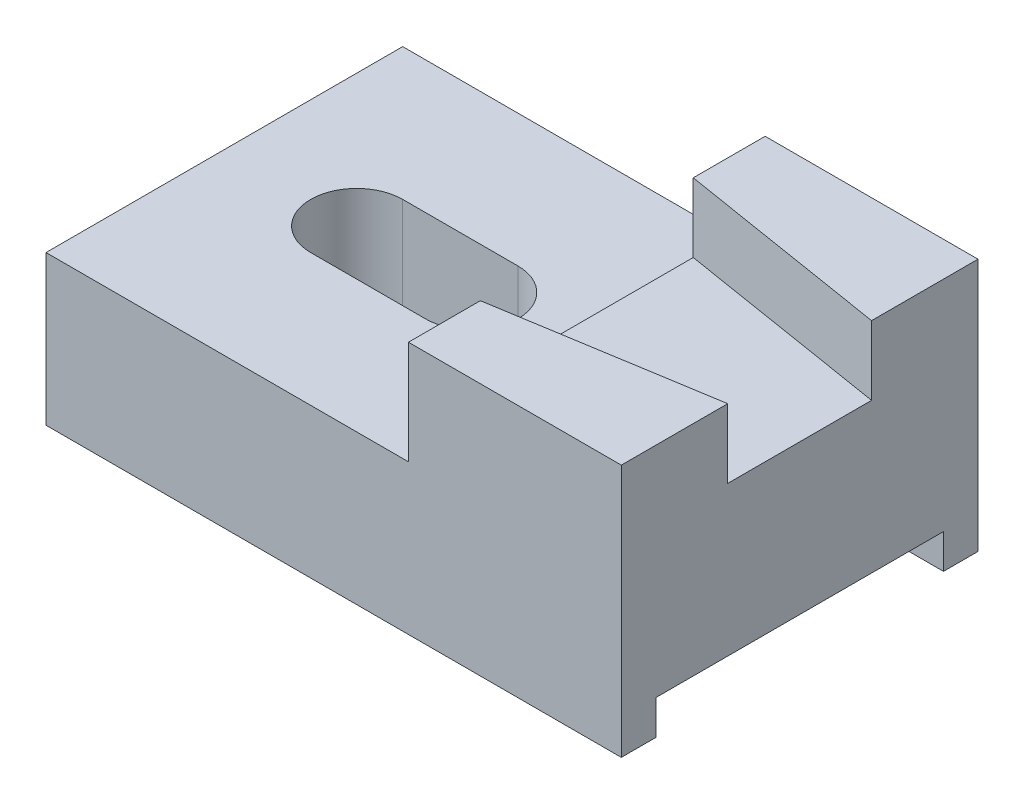
ISO-10303-21;
HEADER;
FILE_DESCRIPTION(('STEP AP214'),'2;1');
FILE_NAME('part.step','',(''),(''),'','','');
FILE_SCHEMA(('AUTOMOTIVE_DESIGN { 1 0 10303 214 1 1 1 1 }'));
ENDSEC;
DATA;
#1=APPLICATION_CONTEXT('core data for automotive mechanical design processes');
#2=APPLICATION_PROTOCOL_DEFINITION('international standard','automotive_design',2000,#1);
#3=PRODUCT_CONTEXT('',#1,'mechanical');
#4=PRODUCT('Part','Part','',(#3));
#5=PRODUCT_RELATED_PRODUCT_CATEGORY('part','',(#4));
#6=PRODUCT_DEFINITION_FORMATION('','',#4);
#7=PRODUCT_DEFINITION_CONTEXT('part definition',#1,'design');
#8=PRODUCT_DEFINITION('design','',#6,#7);
#9=PRODUCT_DEFINITION_SHAPE('','',#8);
#10=(LENGTH_UNIT() NAMED_UNIT(*) SI_UNIT(.MILLI.,.METRE.));
#11=(NAMED_UNIT(*) PLANE_ANGLE_UNIT() SI_UNIT($,.RADIAN.));
#12=(NAMED_UNIT(*) SI_UNIT($,.STERADIAN.) SOLID_ANGLE_UNIT());
#13=UNCERTAINTY_MEASURE_WITH_UNIT(LENGTH_MEASURE(1.E-05),#10,'distance_accuracy_value','');
#14=(GEOMETRIC_REPRESENTATION_CONTEXT(3) GLOBAL_UNCERTAINTY_ASSIGNED_CONTEXT((#13)) GLOBAL_UNIT_ASSIGNED_CONTEXT((#10,
#11,#12)) REPRESENTATION_CONTEXT('',''));
#15=CARTESIAN_POINT('',(0.,0.,0.));
#16=DIRECTION('',(0.,0.,1.));
#17=DIRECTION('',(1.,0.,0.));
#18=AXIS2_PLACEMENT_3D('',#15,#16,#17);
#19=CARTESIAN_POINT('',(100.,0.,31.));
#20=DIRECTION('',(0.,1.,0.));
#21=DIRECTION('',(0.,0.,1.));
#22=AXIS2_PLACEMENT_3D('',#19,#20,#21);
#23=PLANE('',#22);
#24=DIRECTION('',(-1.,0.,0.));
#25=VECTOR('',#24,1.);
#26=CARTESIAN_POINT('',(100.,0.,-25.));
#27=LINE('',#26,#25);
#28=CARTESIAN_POINT('',(100.,0.,-25.));
#29=VERTEX_POINT('',#28);
#30=CARTESIAN_POINT('',(0.,0.,-25.));
#31=VERTEX_POINT('',#30);
#32=EDGE_CURVE('E166',#29,#31,#27,.T.);
#33=ORIENTED_EDGE('',*,*,#32,.T.);
#34=DIRECTION('',(0.,0.,-1.));
#35=VECTOR('',#34,1.);
#36=CARTESIAN_POINT('',(0.,0.,31.));
#37=LINE('',#36,#35);
#38=CARTESIAN_POINT('',(0.,0.,-31.));
#39=VERTEX_POINT('',#38);
#40=EDGE_CURVE('E265',#31,#39,#37,.T.);
#41=ORIENTED_EDGE('',*,*,#40,.T.);
#42=DIRECTION('',(1.,0.,0.));
#43=VECTOR('',#42,1.);
#44=CARTESIAN_POINT('',(100.,0.,-31.));
#45=LINE('',#44,#43);
#46=CARTESIAN_POINT('',(100.,0.,-31.));
#47=VERTEX_POINT('',#46);
#48=EDGE_CURVE('E241',#39,#47,#45,.T.);
#49=ORIENTED_EDGE('',*,*,#48,.T.);
#50=DIRECTION('',(0.,0.,-1.));
#51=VECTOR('',#50,1.);
#52=CARTESIAN_POINT('',(100.,0.,31.));
#53=LINE('',#52,#51);
#54=EDGE_CURVE('E291',#29,#47,#53,.T.);
#55=ORIENTED_EDGE('',*,*,#54,.F.);
#56=EDGE_LOOP('',(#33,#41,#49,#55));
#57=FACE_BOUND('',#56,.T.);
#58=ADVANCED_FACE('F39',(#57),#23,.F.);
#59=DIRECTION('',(-1.,0.,0.));
#60=VECTOR('',#59,1.);
#61=CARTESIAN_POINT('',(100.,0.,25.));
#62=LINE('',#61,#60);
#63=CARTESIAN_POINT('',(100.,0.,25.));
#64=VERTEX_POINT('',#63);
#65=CARTESIAN_POINT('',(0.,0.,25.));
#66=VERTEX_POINT('',#65);
#67=EDGE_CURVE('E52',#64,#66,#62,.T.);
#68=ORIENTED_EDGE('',*,*,#67,.F.);
#69=CARTESIAN_POINT('',(100.,0.,31.));
#70=VERTEX_POINT('',#69);
#71=EDGE_CURVE('E46',#70,#64,#53,.T.);
#72=ORIENTED_EDGE('',*,*,#71,.F.);
#73=DIRECTION('',(1.,0.,0.));
#74=VECTOR('',#73,1.);
#75=CARTESIAN_POINT('',(100.,0.,31.));
#76=LINE('',#75,#74);
#77=CARTESIAN_POINT('',(0.,0.,31.));
#78=VERTEX_POINT('',#77);
#79=EDGE_CURVE('E246',#78,#70,#76,.T.);
#80=ORIENTED_EDGE('',*,*,#79,.F.);
#81=EDGE_CURVE('E280',#78,#66,#37,.T.);
#82=ORIENTED_EDGE('',*,*,#81,.T.);
#83=EDGE_LOOP('',(#68,#72,#80,#82));
#84=FACE_BOUND('',#83,.T.);
#85=ADVANCED_FACE('F341',(#84),#23,.F.);
#86=CARTESIAN_POINT('',(100.,44.,31.));
#87=DIRECTION('',(-1.,0.,0.));
#88=DIRECTION('',(0.,0.,1.));
#89=AXIS2_PLACEMENT_3D('',#86,#87,#88);
#90=PLANE('',#89);
#91=DIRECTION('',(0.,1.,0.));
#92=VECTOR('',#91,1.);
#93=CARTESIAN_POINT('',(100.,0.,-25.));
#94=LINE('',#93,#92);
#95=CARTESIAN_POINT('',(100.,5.99999999999997,-25.));
#96=VERTEX_POINT('',#95);
#97=EDGE_CURVE('E162',#29,#96,#94,.T.);
#98=ORIENTED_EDGE('',*,*,#97,.F.);
#99=ORIENTED_EDGE('',*,*,#54,.T.);
#100=DIRECTION('',(0.,1.,0.));
#101=VECTOR('',#100,1.);
#102=CARTESIAN_POINT('',(100.,44.,-31.));
#103=LINE('',#102,#101);
#104=CARTESIAN_POINT('',(100.,44.,-31.));
#105=VERTEX_POINT('',#104);
#106=EDGE_CURVE('E264',#47,#105,#103,.T.);
#107=ORIENTED_EDGE('',*,*,#106,.T.);
#108=DIRECTION('',(0.,0.,-1.));
#109=VECTOR('',#108,1.);
#110=CARTESIAN_POINT('',(100.,44.,31.));
#111=LINE('',#110,#109);
#112=CARTESIAN_POINT('',(100.,44.,-12.5));
#113=VERTEX_POINT('',#112);
#114=EDGE_CURVE('E287',#113,#105,#111,.T.);
#115=ORIENTED_EDGE('',*,*,#114,.F.);
#116=DIRECTION('',(0.,1.,0.));
#117=VECTOR('',#116,1.);
#118=CARTESIAN_POINT('',(100.,32.,-12.5));
#119=LINE('',#118,#117);
#120=CARTESIAN_POINT('',(100.,32.,-12.5));
#121=VERTEX_POINT('',#120);
#122=EDGE_CURVE('E217',#121,#113,#119,.T.);
#123=ORIENTED_EDGE('',*,*,#122,.F.);
#124=DIRECTION('',(0.,0.,-1.));
#125=VECTOR('',#124,1.);
#126=CARTESIAN_POINT('',(100.,32.,-12.5));
#127=LINE('',#126,#125);
#128=CARTESIAN_POINT('',(100.,32.,12.5));
#129=VERTEX_POINT('',#128);
#130=EDGE_CURVE('E215',#129,#121,#127,.T.);
#131=ORIENTED_EDGE('',*,*,#130,.F.);
#132=DIRECTION('',(0.,1.,0.));
#133=VECTOR('',#132,1.);
#134=CARTESIAN_POINT('',(100.,32.,12.5));
#135=LINE('',#134,#133);
#136=CARTESIAN_POINT('',(100.,44.,12.5));
#137=VERTEX_POINT('',#136);
#138=EDGE_CURVE('E222',#129,#137,#135,.T.);
#139=ORIENTED_EDGE('',*,*,#138,.T.);
#140=CARTESIAN_POINT('',(100.,44.,31.));
#141=VERTEX_POINT('',#140);
#142=EDGE_CURVE('E292',#141,#137,#111,.T.);
#143=ORIENTED_EDGE('',*,*,#142,.F.);
#144=DIRECTION('',(0.,1.,0.));
#145=VECTOR('',#144,1.);
#146=CARTESIAN_POINT('',(100.,44.,31.));
#147=LINE('',#146,#145);
#148=EDGE_CURVE('E253',#70,#141,#147,.T.);
#149=ORIENTED_EDGE('',*,*,#148,.F.);
#150=ORIENTED_EDGE('',*,*,#71,.T.);
#151=DIRECTION('',(0.,-1.,0.));
#152=VECTOR('',#151,1.);
#153=CARTESIAN_POINT('',(100.,5.99999999999997,25.));
#154=LINE('',#153,#152);
#155=CARTESIAN_POINT('',(100.,5.99999999999997,25.));
#156=VERTEX_POINT('',#155);
#157=EDGE_CURVE('E186',#156,#64,#154,.T.);
#158=ORIENTED_EDGE('',*,*,#157,.F.);
#159=DIRECTION('',(0.,0.,1.));
#160=VECTOR('',#159,1.);
#161=CARTESIAN_POINT('',(100.,5.99999999999997,-25.));
#162=LINE('',#161,#160);
#163=EDGE_CURVE('E175',#96,#156,#162,.T.);
#164=ORIENTED_EDGE('',*,*,#163,.F.);
#165=EDGE_LOOP('',(#98,#99,#107,#115,#123,#131,#139,#143,#149,#150,#158,#164));
#166=FACE_BOUND('',#165,.T.);
#167=ADVANCED_FACE('F183',(#166),#90,.F.);
#168=CARTESIAN_POINT('',(0.,0.,31.));
#169=DIRECTION('',(1.,0.,0.));
#170=DIRECTION('',(0.,1.,0.));
#171=AXIS2_PLACEMENT_3D('',#168,#169,#170);
#172=PLANE('',#171);
#173=DIRECTION('',(0.,1.,0.));
#174=VECTOR('',#173,1.);
#175=CARTESIAN_POINT('',(0.,0.,-25.));
#176=LINE('',#175,#174);
#177=CARTESIAN_POINT('',(0.,5.99999999999999,-25.));
#178=VERTEX_POINT('',#177);
#179=EDGE_CURVE('E193',#31,#178,#176,.T.);
#180=ORIENTED_EDGE('',*,*,#179,.T.);
#181=DIRECTION('',(0.,0.,1.));
#182=VECTOR('',#181,1.);
#183=CARTESIAN_POINT('',(0.,5.99999999999999,-25.));
#184=LINE('',#183,#182);
#185=CARTESIAN_POINT('',(0.,5.99999999999999,25.));
#186=VERTEX_POINT('',#185);
#187=EDGE_CURVE('E177',#178,#186,#184,.T.);
#188=ORIENTED_EDGE('',*,*,#187,.T.);
#189=DIRECTION('',(0.,-1.,0.));
#190=VECTOR('',#189,1.);
#191=CARTESIAN_POINT('',(0.,5.99999999999999,25.));
#192=LINE('',#191,#190);
#193=EDGE_CURVE('E173',#186,#66,#192,.T.);
#194=ORIENTED_EDGE('',*,*,#193,.T.);
#195=ORIENTED_EDGE('',*,*,#81,.F.);
#196=DIRECTION('',(0.,-1.,0.));
#197=VECTOR('',#196,1.);
#198=CARTESIAN_POINT('',(0.,0.,31.));
#199=LINE('',#198,#197);
#200=CARTESIAN_POINT('',(0.,26.,31.));
#201=VERTEX_POINT('',#200);
#202=EDGE_CURVE('E257',#201,#78,#199,.T.);
#203=ORIENTED_EDGE('',*,*,#202,.F.);
#204=DIRECTION('',(0.,0.,-1.));
#205=VECTOR('',#204,1.);
#206=CARTESIAN_POINT('',(0.,26.,31.));
#207=LINE('',#206,#205);
#208=CARTESIAN_POINT('',(0.,26.,-31.));
#209=VERTEX_POINT('',#208);
#210=EDGE_CURVE('E278',#201,#209,#207,.T.);
#211=ORIENTED_EDGE('',*,*,#210,.T.);
#212=DIRECTION('',(0.,-1.,0.));
#213=VECTOR('',#212,1.);
#214=CARTESIAN_POINT('',(0.,0.,-31.));
#215=LINE('',#214,#213);
#216=EDGE_CURVE('E252',#209,#39,#215,.T.);
#217=ORIENTED_EDGE('',*,*,#216,.T.);
#218=ORIENTED_EDGE('',*,*,#40,.F.);
#219=EDGE_LOOP('',(#180,#188,#194,#195,#203,#211,#217,#218));
#220=FACE_BOUND('',#219,.T.);
#221=ADVANCED_FACE('F308',(#220),#172,.F.);
#222=CARTESIAN_POINT('',(23.,-36.,0.));
#223=DIRECTION('',(0.,1.,0.));
#224=DIRECTION('',(0.,0.,1.));
#225=AXIS2_PLACEMENT_3D('',#222,#223,#224);
#226=CYLINDRICAL_SURFACE('',#225,8.);
#227=CARTESIAN_POINT('',(23.,5.99999999999998,0.));
#228=DIRECTION('',(0.,-1.,0.));
#229=DIRECTION('',(1.,0.,0.));
#230=AXIS2_PLACEMENT_3D('',#227,#228,#229);
#231=CIRCLE('',#230,8.);
#232=CARTESIAN_POINT('',(23.,5.99999999999998,-8.));
#233=VERTEX_POINT('',#232);
#234=CARTESIAN_POINT('',(23.,5.99999999999998,8.));
#235=VERTEX_POINT('',#234);
#236=EDGE_CURVE('E58',#233,#235,#231,.F.);
#237=ORIENTED_EDGE('',*,*,#236,.F.);
#238=DIRECTION('',(0.,1.,0.));
#239=VECTOR('',#238,1.);
#240=CARTESIAN_POINT('',(23.,-36.,-8.));
#241=LINE('',#240,#239);
#242=CARTESIAN_POINT('',(23.,26.,-8.));
#243=VERTEX_POINT('',#242);
#244=EDGE_CURVE('E238',#233,#243,#241,.T.);
#245=ORIENTED_EDGE('',*,*,#244,.T.);
#246=CARTESIAN_POINT('',(23.,26.,0.));
#247=DIRECTION('',(0.,1.,0.));
#248=DIRECTION('',(0.,0.,1.));
#249=AXIS2_PLACEMENT_3D('',#246,#247,#248);
#250=CIRCLE('',#249,8.);
#251=CARTESIAN_POINT('',(23.,26.,8.));
#252=VERTEX_POINT('',#251);
#253=EDGE_CURVE('E219',#243,#252,#250,.T.);
#254=ORIENTED_EDGE('',*,*,#253,.T.);
#255=DIRECTION('',(0.,1.,0.));
#256=VECTOR('',#255,1.);
#257=CARTESIAN_POINT('',(23.,-36.,8.));
#258=LINE('',#257,#256);
#259=EDGE_CURVE('E239',#235,#252,#258,.T.);
#260=ORIENTED_EDGE('',*,*,#259,.F.);
#261=EDGE_LOOP('',(#237,#245,#254,#260));
#262=FACE_BOUND('',#261,.T.);
#263=ADVANCED_FACE('F361',(#262),#226,.F.);
#264=CARTESIAN_POINT('',(23.,-36.,-8.));
#265=DIRECTION('',(0.,0.,-1.));
#266=DIRECTION('',(-1.,0.,0.));
#267=AXIS2_PLACEMENT_3D('',#264,#265,#266);
#268=PLANE('',#267);
#269=DIRECTION('',(-1.,0.,0.));
#270=VECTOR('',#269,1.);
#271=CARTESIAN_POINT('',(23.,5.99999999999998,-8.));
#272=LINE('',#271,#270);
#273=CARTESIAN_POINT('',(43.,5.99999999999998,-8.));
#274=VERTEX_POINT('',#273);
#275=EDGE_CURVE('E200',#274,#233,#272,.T.);
#276=ORIENTED_EDGE('',*,*,#275,.F.);
#277=DIRECTION('',(0.,1.,0.));
#278=VECTOR('',#277,1.);
#279=CARTESIAN_POINT('',(43.,-36.,-8.));
#280=LINE('',#279,#278);
#281=CARTESIAN_POINT('',(43.,26.,-8.));
#282=VERTEX_POINT('',#281);
#283=EDGE_CURVE('E245',#274,#282,#280,.T.);
#284=ORIENTED_EDGE('',*,*,#283,.T.);
#285=DIRECTION('',(-1.,0.,0.));
#286=VECTOR('',#285,1.);
#287=CARTESIAN_POINT('',(23.,26.,-8.));
#288=LINE('',#287,#286);
#289=EDGE_CURVE('E237',#282,#243,#288,.T.);
#290=ORIENTED_EDGE('',*,*,#289,.T.);
#291=ORIENTED_EDGE('',*,*,#244,.F.);
#292=EDGE_LOOP('',(#276,#284,#290,#291));
#293=FACE_BOUND('',#292,.T.);
#294=ADVANCED_FACE('F377',(#293),#268,.F.);
#295=CARTESIAN_POINT('',(43.,-36.,0.));
#296=DIRECTION('',(0.,1.,0.));
#297=DIRECTION('',(0.,0.,1.));
#298=AXIS2_PLACEMENT_3D('',#295,#296,#297);
#299=CYLINDRICAL_SURFACE('',#298,8.);
#300=CARTESIAN_POINT('',(43.,5.99999999999998,0.));
#301=DIRECTION('',(0.,-1.,0.));
#302=DIRECTION('',(1.,0.,0.));
#303=AXIS2_PLACEMENT_3D('',#300,#301,#302);
#304=CIRCLE('',#303,8.);
#305=CARTESIAN_POINT('',(43.,5.99999999999998,8.));
#306=VERTEX_POINT('',#305);
#307=EDGE_CURVE('E182',#306,#274,#304,.F.);
#308=ORIENTED_EDGE('',*,*,#307,.F.);
#309=DIRECTION('',(0.,1.,0.));
#310=VECTOR('',#309,1.);
#311=CARTESIAN_POINT('',(43.,-36.,8.));
#312=LINE('',#311,#310);
#313=CARTESIAN_POINT('',(43.,26.,8.));
#314=VERTEX_POINT('',#313);
#315=EDGE_CURVE('E242',#306,#314,#312,.T.);
#316=ORIENTED_EDGE('',*,*,#315,.T.);
#317=CARTESIAN_POINT('',(43.,26.,0.));
#318=DIRECTION('',(0.,1.,0.));
#319=DIRECTION('',(0.,0.,1.));
#320=AXIS2_PLACEMENT_3D('',#317,#318,#319);
#321=CIRCLE('',#320,8.);
#322=EDGE_CURVE('E231',#314,#282,#321,.T.);
#323=ORIENTED_EDGE('',*,*,#322,.T.);
#324=ORIENTED_EDGE('',*,*,#283,.F.);
#325=EDGE_LOOP('',(#308,#316,#323,#324));
#326=FACE_BOUND('',#325,.T.);
#327=ADVANCED_FACE('F383',(#326),#299,.F.);
#328=CARTESIAN_POINT('',(23.,-36.,8.));
#329=DIRECTION('',(0.,0.,1.));
#330=DIRECTION('',(1.,0.,0.));
#331=AXIS2_PLACEMENT_3D('',#328,#329,#330);
#332=PLANE('',#331);
#333=DIRECTION('',(1.,0.,0.));
#334=VECTOR('',#333,1.);
#335=CARTESIAN_POINT('',(23.,5.99999999999998,8.));
#336=LINE('',#335,#334);
#337=EDGE_CURVE('E11',#235,#306,#336,.T.);
#338=ORIENTED_EDGE('',*,*,#337,.F.);
#339=ORIENTED_EDGE('',*,*,#259,.T.);
#340=DIRECTION('',(1.,0.,0.));
#341=VECTOR('',#340,1.);
#342=CARTESIAN_POINT('',(23.,26.,8.));
#343=LINE('',#342,#341);
#344=EDGE_CURVE('E227',#252,#314,#343,.T.);
#345=ORIENTED_EDGE('',*,*,#344,.T.);
#346=ORIENTED_EDGE('',*,*,#315,.F.);
#347=EDGE_LOOP('',(#338,#339,#345,#346));
#348=FACE_BOUND('',#347,.T.);
#349=ADVANCED_FACE('F381',(#348),#332,.F.);
#350=CARTESIAN_POINT('',(63.,44.,31.));
#351=DIRECTION('',(0.,-1.,0.));
#352=DIRECTION('',(1.,0.,0.));
#353=AXIS2_PLACEMENT_3D('',#350,#351,#352);
#354=PLANE('',#353);
#355=DIRECTION('',(0.,0.,-1.));
#356=VECTOR('',#355,1.);
#357=CARTESIAN_POINT('',(63.,44.,31.));
#358=LINE('',#357,#356);
#359=CARTESIAN_POINT('',(63.,44.,-18.5));
#360=VERTEX_POINT('',#359);
#361=CARTESIAN_POINT('',(63.,44.,-31.));
#362=VERTEX_POINT('',#361);
#363=EDGE_CURVE('E288',#360,#362,#358,.T.);
#364=ORIENTED_EDGE('',*,*,#363,.F.);
#365=DIRECTION('',(-0.987105477747585,0.,-0.160071158553662));
#366=VECTOR('',#365,1.);
#367=CARTESIAN_POINT('',(63.,44.,-18.5));
#368=LINE('',#367,#366);
#369=EDGE_CURVE('E205',#113,#360,#368,.T.);
#370=ORIENTED_EDGE('',*,*,#369,.F.);
#371=ORIENTED_EDGE('',*,*,#114,.T.);
#372=DIRECTION('',(-1.,0.,0.));
#373=VECTOR('',#372,1.);
#374=CARTESIAN_POINT('',(63.,44.,-31.));
#375=LINE('',#374,#373);
#376=EDGE_CURVE('E268',#105,#362,#375,.T.);
#377=ORIENTED_EDGE('',*,*,#376,.T.);
#378=EDGE_LOOP('',(#364,#370,#371,#377));
#379=FACE_BOUND('',#378,.T.);
#380=ADVANCED_FACE('F325',(#379),#354,.F.);
#381=ORIENTED_EDGE('',*,*,#142,.T.);
#382=DIRECTION('',(0.987105477747585,0.,-0.160071158553662));
#383=VECTOR('',#382,1.);
#384=CARTESIAN_POINT('',(63.,44.,18.5));
#385=LINE('',#384,#383);
#386=CARTESIAN_POINT('',(63.,44.,18.5));
#387=VERTEX_POINT('',#386);
#388=EDGE_CURVE('E206',#387,#137,#385,.T.);
#389=ORIENTED_EDGE('',*,*,#388,.F.);
#390=CARTESIAN_POINT('',(63.,44.,31.));
#391=VERTEX_POINT('',#390);
#392=EDGE_CURVE('E290',#391,#387,#358,.T.);
#393=ORIENTED_EDGE('',*,*,#392,.F.);
#394=DIRECTION('',(-1.,0.,0.));
#395=VECTOR('',#394,1.);
#396=CARTESIAN_POINT('',(63.,44.,31.));
#397=LINE('',#396,#395);
#398=EDGE_CURVE('E255',#141,#391,#397,.T.);
#399=ORIENTED_EDGE('',*,*,#398,.F.);
#400=EDGE_LOOP('',(#381,#389,#393,#399));
#401=FACE_BOUND('',#400,.T.);
#402=ADVANCED_FACE('F339',(#401),#354,.F.);
#403=CARTESIAN_POINT('',(63.,26.,31.));
#404=DIRECTION('',(1.,0.,0.));
#405=DIRECTION('',(0.,1.,0.));
#406=AXIS2_PLACEMENT_3D('',#403,#404,#405);
#407=PLANE('',#406);
#408=DIRECTION('',(0.,0.,1.));
#409=VECTOR('',#408,1.);
#410=CARTESIAN_POINT('',(63.,32.,-18.5));
#411=LINE('',#410,#409);
#412=CARTESIAN_POINT('',(63.,32.,-18.5));
#413=VERTEX_POINT('',#412);
#414=CARTESIAN_POINT('',(63.,32.,18.5));
#415=VERTEX_POINT('',#414);
#416=EDGE_CURVE('E202',#413,#415,#411,.T.);
#417=ORIENTED_EDGE('',*,*,#416,.F.);
#418=DIRECTION('',(0.,1.,0.));
#419=VECTOR('',#418,1.);
#420=CARTESIAN_POINT('',(63.,32.,-18.5));
#421=LINE('',#420,#419);
#422=EDGE_CURVE('E214',#413,#360,#421,.T.);
#423=ORIENTED_EDGE('',*,*,#422,.T.);
#424=ORIENTED_EDGE('',*,*,#363,.T.);
#425=DIRECTION('',(0.,-1.,0.));
#426=VECTOR('',#425,1.);
#427=CARTESIAN_POINT('',(63.,26.,-31.));
#428=LINE('',#427,#426);
#429=CARTESIAN_POINT('',(63.,26.,-31.));
#430=VERTEX_POINT('',#429);
#431=EDGE_CURVE('E271',#362,#430,#428,.T.);
#432=ORIENTED_EDGE('',*,*,#431,.T.);
#433=DIRECTION('',(0.,0.,-1.));
#434=VECTOR('',#433,1.);
#435=CARTESIAN_POINT('',(63.,26.,31.));
#436=LINE('',#435,#434);
#437=CARTESIAN_POINT('',(63.,26.,31.));
#438=VERTEX_POINT('',#437);
#439=EDGE_CURVE('E285',#438,#430,#436,.T.);
#440=ORIENTED_EDGE('',*,*,#439,.F.);
#441=DIRECTION('',(0.,-1.,0.));
#442=VECTOR('',#441,1.);
#443=CARTESIAN_POINT('',(63.,26.,31.));
#444=LINE('',#443,#442);
#445=EDGE_CURVE('E258',#391,#438,#444,.T.);
#446=ORIENTED_EDGE('',*,*,#445,.F.);
#447=ORIENTED_EDGE('',*,*,#392,.T.);
#448=DIRECTION('',(0.,1.,0.));
#449=VECTOR('',#448,1.);
#450=CARTESIAN_POINT('',(63.,32.,18.5));
#451=LINE('',#450,#449);
#452=EDGE_CURVE('E221',#415,#387,#451,.T.);
#453=ORIENTED_EDGE('',*,*,#452,.F.);
#454=EDGE_LOOP('',(#417,#423,#424,#432,#440,#446,#447,#453));
#455=FACE_BOUND('',#454,.T.);
#456=ADVANCED_FACE('F320',(#455),#407,.F.);
#457=CARTESIAN_POINT('',(0.,26.,31.));
#458=DIRECTION('',(0.,-1.,0.));
#459=DIRECTION('',(0.,0.,-1.));
#460=AXIS2_PLACEMENT_3D('',#457,#458,#459);
#461=PLANE('',#460);
#462=ORIENTED_EDGE('',*,*,#344,.F.);
#463=ORIENTED_EDGE('',*,*,#253,.F.);
#464=ORIENTED_EDGE('',*,*,#289,.F.);
#465=ORIENTED_EDGE('',*,*,#322,.F.);
#466=EDGE_LOOP('',(#462,#463,#464,#465));
#467=FACE_BOUND('',#466,.T.);
#468=DIRECTION('',(-1.,0.,0.));
#469=VECTOR('',#468,1.);
#470=CARTESIAN_POINT('',(0.,26.,-31.));
#471=LINE('',#470,#469);
#472=EDGE_CURVE('E272',#430,#209,#471,.T.);
#473=ORIENTED_EDGE('',*,*,#472,.T.);
#474=ORIENTED_EDGE('',*,*,#210,.F.);
#475=DIRECTION('',(-1.,0.,0.));
#476=VECTOR('',#475,1.);
#477=CARTESIAN_POINT('',(0.,26.,31.));
#478=LINE('',#477,#476);
#479=EDGE_CURVE('E256',#438,#201,#478,.T.);
#480=ORIENTED_EDGE('',*,*,#479,.F.);
#481=ORIENTED_EDGE('',*,*,#439,.T.);
#482=EDGE_LOOP('',(#473,#474,#480,#481));
#483=FACE_BOUND('',#482,.T.);
#484=ADVANCED_FACE('F313',(#467,#483),#461,.F.);
#485=CARTESIAN_POINT('',(0.,0.,31.));
#486=DIRECTION('',(0.,0.,-1.));
#487=DIRECTION('',(-1.,0.,0.));
#488=AXIS2_PLACEMENT_3D('',#485,#486,#487);
#489=PLANE('',#488);
#490=ORIENTED_EDGE('',*,*,#79,.T.);
#491=ORIENTED_EDGE('',*,*,#148,.T.);
#492=ORIENTED_EDGE('',*,*,#398,.T.);
#493=ORIENTED_EDGE('',*,*,#445,.T.);
#494=ORIENTED_EDGE('',*,*,#479,.T.);
#495=ORIENTED_EDGE('',*,*,#202,.T.);
#496=EDGE_LOOP('',(#490,#491,#492,#493,#494,#495));
#497=FACE_BOUND('',#496,.T.);
#498=ADVANCED_FACE('F338',(#497),#489,.F.);
#499=CARTESIAN_POINT('',(0.,0.,-31.));
#500=DIRECTION('',(0.,0.,-1.));
#501=DIRECTION('',(-1.,0.,0.));
#502=AXIS2_PLACEMENT_3D('',#499,#500,#501);
#503=PLANE('',#502);
#504=ORIENTED_EDGE('',*,*,#48,.F.);
#505=ORIENTED_EDGE('',*,*,#216,.F.);
#506=ORIENTED_EDGE('',*,*,#472,.F.);
#507=ORIENTED_EDGE('',*,*,#431,.F.);
#508=ORIENTED_EDGE('',*,*,#376,.F.);
#509=ORIENTED_EDGE('',*,*,#106,.F.);
#510=EDGE_LOOP('',(#504,#505,#506,#507,#508,#509));
#511=FACE_BOUND('',#510,.T.);
#512=ADVANCED_FACE('F303',(#511),#503,.T.);
#513=CARTESIAN_POINT('',(63.,32.,-18.5));
#514=DIRECTION('',(0.160071158553662,0.,-0.987105477747585));
#515=DIRECTION('',(-0.987105477747585,0.,-0.160071158553662));
#516=AXIS2_PLACEMENT_3D('',#513,#514,#515);
#517=PLANE('',#516);
#518=ORIENTED_EDGE('',*,*,#369,.T.);
#519=ORIENTED_EDGE('',*,*,#422,.F.);
#520=DIRECTION('',(-0.987105477747585,0.,-0.160071158553662));
#521=VECTOR('',#520,1.);
#522=CARTESIAN_POINT('',(63.,32.,-18.5));
#523=LINE('',#522,#521);
#524=EDGE_CURVE('E201',#121,#413,#523,.T.);
#525=ORIENTED_EDGE('',*,*,#524,.F.);
#526=ORIENTED_EDGE('',*,*,#122,.T.);
#527=EDGE_LOOP('',(#518,#519,#525,#526));
#528=FACE_BOUND('',#527,.T.);
#529=ADVANCED_FACE('F326',(#528),#517,.F.);
#530=CARTESIAN_POINT('',(63.,32.,18.5));
#531=DIRECTION('',(0.160071158553662,0.,0.987105477747585));
#532=DIRECTION('',(0.987105477747585,0.,-0.160071158553662));
#533=AXIS2_PLACEMENT_3D('',#530,#531,#532);
#534=PLANE('',#533);
#535=ORIENTED_EDGE('',*,*,#388,.T.);
#536=ORIENTED_EDGE('',*,*,#138,.F.);
#537=DIRECTION('',(0.987105477747585,0.,-0.160071158553662));
#538=VECTOR('',#537,1.);
#539=CARTESIAN_POINT('',(63.,32.,18.5));
#540=LINE('',#539,#538);
#541=EDGE_CURVE('E207',#415,#129,#540,.T.);
#542=ORIENTED_EDGE('',*,*,#541,.F.);
#543=ORIENTED_EDGE('',*,*,#452,.T.);
#544=EDGE_LOOP('',(#535,#536,#542,#543));
#545=FACE_BOUND('',#544,.T.);
#546=ADVANCED_FACE('F332',(#545),#534,.F.);
#547=CARTESIAN_POINT('',(0.,32.,0.));
#548=DIRECTION('',(0.,-1.,0.));
#549=DIRECTION('',(1.,0.,0.));
#550=AXIS2_PLACEMENT_3D('',#547,#548,#549);
#551=PLANE('',#550);
#552=ORIENTED_EDGE('',*,*,#524,.T.);
#553=ORIENTED_EDGE('',*,*,#416,.T.);
#554=ORIENTED_EDGE('',*,*,#541,.T.);
#555=ORIENTED_EDGE('',*,*,#130,.T.);
#556=EDGE_LOOP('',(#552,#553,#554,#555));
#557=FACE_BOUND('',#556,.T.);
#558=ADVANCED_FACE('F327',(#557),#551,.F.);
#559=CARTESIAN_POINT('',(100.,5.99999999999997,-25.));
#560=DIRECTION('',(0.,-1.,0.));
#561=DIRECTION('',(1.,0.,0.));
#562=AXIS2_PLACEMENT_3D('',#559,#560,#561);
#563=PLANE('',#562);
#564=ORIENTED_EDGE('',*,*,#187,.F.);
#565=DIRECTION('',(-1.,0.,0.));
#566=VECTOR('',#565,1.);
#567=CARTESIAN_POINT('',(100.,5.99999999999997,-25.));
#568=LINE('',#567,#566);
#569=EDGE_CURVE('E167',#96,#178,#568,.T.);
#570=ORIENTED_EDGE('',*,*,#569,.F.);
#571=ORIENTED_EDGE('',*,*,#163,.T.);
#572=DIRECTION('',(-1.,0.,0.));
#573=VECTOR('',#572,1.);
#574=CARTESIAN_POINT('',(100.,5.99999999999997,25.));
#575=LINE('',#574,#573);
#576=EDGE_CURVE('E185',#156,#186,#575,.T.);
#577=ORIENTED_EDGE('',*,*,#576,.T.);
#578=EDGE_LOOP('',(#564,#570,#571,#577));
#579=FACE_BOUND('',#578,.T.);
#580=ORIENTED_EDGE('',*,*,#236,.T.);
#581=ORIENTED_EDGE('',*,*,#337,.T.);
#582=ORIENTED_EDGE('',*,*,#307,.T.);
#583=ORIENTED_EDGE('',*,*,#275,.T.);
#584=EDGE_LOOP('',(#580,#581,#582,#583));
#585=FACE_BOUND('',#584,.T.);
#586=ADVANCED_FACE('F180',(#579,#585),#563,.T.);
#587=CARTESIAN_POINT('',(100.,0.,-25.));
#588=DIRECTION('',(0.,0.,1.));
#589=DIRECTION('',(1.,0.,0.));
#590=AXIS2_PLACEMENT_3D('',#587,#588,#589);
#591=PLANE('',#590);
#592=ORIENTED_EDGE('',*,*,#179,.F.);
#593=ORIENTED_EDGE('',*,*,#32,.F.);
#594=ORIENTED_EDGE('',*,*,#97,.T.);
#595=ORIENTED_EDGE('',*,*,#569,.T.);
#596=EDGE_LOOP('',(#592,#593,#594,#595));
#597=FACE_BOUND('',#596,.T.);
#598=ADVANCED_FACE('F164',(#597),#591,.T.);
#599=CARTESIAN_POINT('',(100.,5.99999999999997,25.));
#600=DIRECTION('',(0.,0.,-1.));
#601=DIRECTION('',(-1.,0.,0.));
#602=AXIS2_PLACEMENT_3D('',#599,#600,#601);
#603=PLANE('',#602);
#604=ORIENTED_EDGE('',*,*,#193,.F.);
#605=ORIENTED_EDGE('',*,*,#576,.F.);
#606=ORIENTED_EDGE('',*,*,#157,.T.);
#607=ORIENTED_EDGE('',*,*,#67,.T.);
#608=EDGE_LOOP('',(#604,#605,#606,#607));
#609=FACE_BOUND('',#608,.T.);
#610=ADVANCED_FACE('F344',(#609),#603,.T.);
#611=CLOSED_SHELL('',(#58,#85,#167,#221,#263,#294,#327,#349,#380,#402,#456,#484,#498,#512,#529,
#546,#558,#586,#598,#610));
#612=MANIFOLD_SOLID_BREP('B2',#611);
#613=ADVANCED_BREP_SHAPE_REPRESENTATION('',(#18,#612),#14);
#614=SHAPE_DEFINITION_REPRESENTATION(#9,#613);
ENDSEC;
END-ISO-10303-21;
